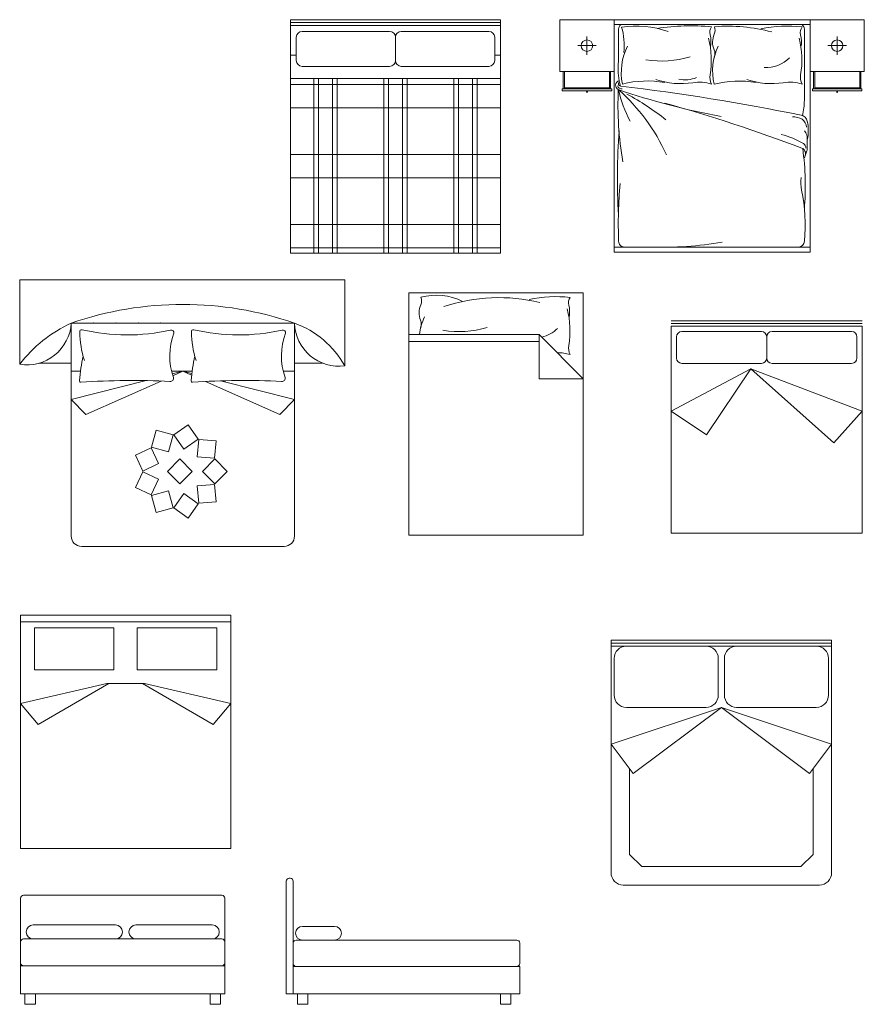
# Model space of a CAD drawing. Units: inches. Extents: x 1994 to 3075, y 3517 to 3950.
# Tile 5 of 58: x 1993.694 to 1993.9789, y 3553.5515 to 3553.8837. Entities that reach past the tile are written whole.
import ezdxf

# ---------------------------------------------------------------- set-up
doc = ezdxf.new("R2010")
doc.units = ezdxf.units.IN
doc.layers.add('A-FURN-REFR', color=8, linetype='Continuous', lineweight=13)

msp = doc.modelspace()

# ---------------------------------------------------------------- linework, layer by layer
at = {"layer": 'A-FURN-REFR'}
for p, q in [((1993.856202557817, 3553.883733619688), (1993.785336416085, 3553.883733619688)), ((1993.785336416085, 3553.804993462208), (1993.785336416085, 3553.883733619688)), ((1993.785336416085, 3553.882749367719), (1993.856202557817, 3553.882749367719)), ((1993.785336416085, 3553.881765115751), (1993.856202557817, 3553.881765115751)), ((1993.856202557817, 3553.883733619688), (1993.856202557817, 3553.804993462208)), ((1993.876219255827, 3553.866219817953), (1993.876219255827, 3553.883730063468)), ((1993.876219255827, 3553.883730063468), (1993.894507734482, 3553.883730063468)), ((1993.894507734482, 3553.883730063474), (1993.960657550884, 3553.883730063461)), ((1993.894507734482, 3553.883730063474), (1993.894507734466, 3553.805323075211)), ((1993.894507734482, 3553.882056862236), (1993.960657550883, 3553.882056862222)), ((1993.960657550884, 3553.883730063461), (1993.960657550867, 3553.805323075197)), ((1993.978946029539, 3553.883730063468), (1993.960657550884, 3553.883730063468)), ((1993.978946029539, 3553.866219817953), (1993.978946029539, 3553.883730063468)), ((1993.787304920022, 3553.869954092129), (1993.787304920022, 3553.877828107877)), ((1993.789273423959, 3553.879796611814), (1993.818800983014, 3553.879796611814)), ((1993.820769486951, 3553.869954092129), (1993.820769486951, 3553.877828107877)), ((1993.822737990888, 3553.879796611814), (1993.852265549944, 3553.879796611814)), ((1993.85423405388, 3553.877828107877), (1993.85423405388, 3553.869954092129)), ((1993.885363495152, 3553.871862008174), (1993.885363495152, 3553.878087873247)), ((1993.958711968042, 3553.85654949402), (1993.958711968047, 3553.880500395955)), ((1993.969801790214, 3553.871862008174), (1993.969801790214, 3553.878087873247)), ((1993.882250562615, 3553.87497494071), (1993.888476427688, 3553.87497494071)), ((1993.97291472275, 3553.87497494071), (1993.966688857678, 3553.87497494071)), ((1993.785336416085, 3553.871779066532), (1993.787304920022, 3553.871779066532)), ((1993.85423405388, 3553.871779066532), (1993.856202557817, 3553.871779066532)), ((1993.789273423959, 3553.867985588192), (1993.818800983014, 3553.867985588192)), ((1993.822737990888, 3553.867985588192), (1993.852265549944, 3553.867985588192)), ((1993.894507734479, 3553.86621981795), (1993.876219255827, 3553.866219817953)), ((1993.877386605528, 3553.866219817953), (1993.877386605527, 3553.860383069447)), ((1993.877775722095, 3553.866219817953), (1993.877775722094, 3553.860383069447)), ((1993.89295126821, 3553.86621981795), (1993.892951268209, 3553.860383069443)), ((1993.893340384778, 3553.86621981795), (1993.893340384776, 3553.860383069443)), ((1993.960657550887, 3553.86621981795), (1993.978946029539, 3553.866219817953)), ((1993.961824900588, 3553.86621981795), (1993.961824900589, 3553.860383069443)), ((1993.962214017155, 3553.86621981795), (1993.962214017156, 3553.860383069443)), ((1993.977389563271, 3553.866219817953), (1993.977389563272, 3553.860383069447)), ((1993.977778679838, 3553.866219817953), (1993.977778679839, 3553.860383069447)), ((1993.785336416085, 3553.863879360431), (1993.856202557817, 3553.863879360431)), ((1993.785336416085, 3553.861910856494), (1993.856202557817, 3553.861910856494)), ((1993.793210431833, 3553.863879360431), (1993.793210431833, 3553.804993462208)), ((1993.794785234983, 3553.863879360431), (1993.794785234983, 3553.804993462208)), ((1993.799509644432, 3553.863879360431), (1993.799509644432, 3553.804993462208)), ((1993.801084447581, 3553.863879360431), (1993.801084447581, 3553.804993462208)), ((1993.816832479078, 3553.863879360431), (1993.816832479078, 3553.804993462208)), ((1993.818407282227, 3553.863879360431), (1993.818407282227, 3553.804993462208)), ((1993.823131691676, 3553.863879360431), (1993.823131691676, 3553.804993462208)), ((1993.824706494825, 3553.863879360431), (1993.824706494825, 3553.804993462208)), ((1993.840454526321, 3553.863879360431), (1993.840454526321, 3553.804993462208)), ((1993.842029329471, 3553.863879360431), (1993.842029329471, 3553.804993462208)), ((1993.84675373892, 3553.863879360431), (1993.84675373892, 3553.804993462208)), ((1993.848328542069, 3553.863879360431), (1993.848328542069, 3553.804993462208)), ((1993.893729501343, 3553.860383069443), (1993.876997488959, 3553.860383069447)), ((1993.876997488959, 3553.860383069447), (1993.876997488959, 3553.859682659626)), ((1993.876997488959, 3553.859682659626), (1993.893729501343, 3553.859682659623)), ((1993.877775722094, 3553.860772186014), (1993.892951268209, 3553.86077218601)), ((1993.893729501343, 3553.859682659623), (1993.893729501343, 3553.860383069443)), ((1993.961435784022, 3553.860383069443), (1993.978167796406, 3553.860383069447)), ((1993.961435784022, 3553.859682659623), (1993.961435784022, 3553.860383069443)), ((1993.978167796406, 3553.859682659626), (1993.961435784022, 3553.859682659623)), ((1993.977389563272, 3553.860772186014), (1993.962214017156, 3553.86077218601)), ((1993.978167796406, 3553.860383069447), (1993.978167796406, 3553.859682659626)), ((1993.785336416085, 3553.854036840746), (1993.856202557817, 3553.854036840746)), ((1993.959684759457, 3553.840101857006), (1993.959684759457, 3553.843919683994)), ((1993.785336416085, 3553.83828880925), (1993.856202557817, 3553.83828880925)), ((1993.959564553778, 3553.83942858826), (1993.958711968038, 3553.83711704396)), ((1993.785336416085, 3553.830414793502), (1993.856202557817, 3553.830414793502)), ((1993.785336416085, 3553.814666762006), (1993.856202557817, 3553.814666762006)), ((1993.785336416085, 3553.806792746258), (1993.856202557817, 3553.806792746258)), ((1993.856202557817, 3553.804993462208), (1993.785336416085, 3553.804993462208)), ((1993.894507734466, 3553.806996276449), (1993.960657550868, 3553.806996276435)), ((1993.894507734466, 3553.805323075211), (1993.960657550867, 3553.805323075197)), ((1993.693977196263, 3553.795927324173), (1993.693977196263, 3553.767437960728)), ((1993.80365945686, 3553.795927324173), (1993.693977196263, 3553.795927324173)), ((1993.80365945686, 3553.795927324173), (1993.80365945686, 3553.76692621804)), ((1993.825218431411, 3553.70978992263), (1993.825218431411, 3553.791608082631)), ((1993.825218431411, 3553.791608082631), (1993.884127555047, 3553.791608082631)), ((1993.884127555047, 3553.791608082631), (1993.884127555047, 3553.70978992263)), ((1993.711353319426, 3553.781334854554), (1993.749029293889, 3553.781334854554)), ((1993.711353319426, 3553.76692621804), (1993.711353319426, 3553.781334854554)), ((1993.786705268352, 3553.781334854554), (1993.749029293889, 3553.781334854554)), ((1993.786705268352, 3553.76692621804), (1993.786705268352, 3553.781334854554)), ((1993.80365945686, 3553.781334854554), (1993.80365945686, 3553.76692621804)), ((1993.978241546912, 3553.782070903671), (1993.913817781701, 3553.782070903671)), ((1993.913817781701, 3553.781176129155), (1993.978241546912, 3553.781176129155)), ((1993.913817781701, 3553.780281354637), (1993.978241546912, 3553.780281354637)), ((1993.913817781701, 3553.710488942325), (1993.913817781701, 3553.780281354637)), ((1993.917396879768, 3553.778491805604), (1993.944240115272, 3553.778491805604)), ((1993.94781921334, 3553.778491805604), (1993.974662448844, 3553.778491805604)), ((1993.978241546912, 3553.780281354637), (1993.978241546912, 3553.710488942325)), ((1993.825218431411, 3553.777469900813), (1993.869203918684, 3553.777469900813)), ((1993.869203918684, 3553.775113537176), (1993.825218431411, 3553.775113537176)), ((1993.884127555047, 3553.762546264449), (1993.869203918684, 3553.777469900813)), ((1993.869203918684, 3553.777469900813), (1993.869203918684, 3553.762546264449)), ((1993.915607330734, 3553.769544060435), (1993.915607330734, 3553.77670225657)), ((1993.946029664306, 3553.769544060435), (1993.946029664306, 3553.77670225657)), ((1993.976451997878, 3553.77670225657), (1993.976451997878, 3553.769544060435)), ((1993.700693126714, 3553.767864459417), (1993.711353319426, 3553.767864459417)), ((1993.711353319426, 3553.709531369957), (1993.711353319426, 3553.76692621804)), ((1993.711353319426, 3553.76507068463), (1993.714474286442, 3553.76507068463)), ((1993.745229054011, 3553.76507068463), (1993.749029293889, 3553.76507068463)), ((1993.749029293889, 3553.76507068463), (1993.74546816915, 3553.764171920895)), ((1993.749029293889, 3553.76507068463), (1993.745653350489, 3553.763563244933)), ((1993.752150260905, 3553.76507068463), (1993.749029293889, 3553.76507068463)), ((1993.749029293889, 3553.76507068463), (1993.752054974805, 3553.764307057271)), ((1993.749029293889, 3553.76507068463), (1993.751991106552, 3553.76374816424)), ((1993.786705268352, 3553.76507068463), (1993.782905028474, 3553.76507068463)), ((1993.786705268352, 3553.767864459417), (1993.796105996925, 3553.767864459417)), ((1993.786705268352, 3553.709531369957), (1993.786705268352, 3553.76692621804)), ((1993.913817781701, 3553.751648570099), (1993.940661017205, 3553.765964962368)), ((1993.917396879768, 3553.767754511401), (1993.944240115272, 3553.767754511401)), ((1993.925706827183, 3553.743673002087), (1993.940661017205, 3553.765964962368)), ((1993.940661017205, 3553.765964962368), (1993.978241546912, 3553.751648570099)), ((1993.940661017205, 3553.765964962368), (1993.968716184927, 3553.740960887158)), ((1993.94781921334, 3553.767754511401), (1993.974662448844, 3553.767754511401)), ((1993.736595982811, 3553.761932740884), (1993.71134319232, 3553.755559391458)), ((1993.741709056693, 3553.761802023153), (1993.716317016293, 3553.750463868108)), ((1993.756653216091, 3553.761666420514), (1993.781741571484, 3553.750463868108)), ((1993.76175885485, 3553.76185797275), (1993.786715395458, 3553.755559391458)), ((1993.869203918684, 3553.762546264449), (1993.884127555047, 3553.762546264449)), ((1993.716317016293, 3553.750463868108), (1993.711353319426, 3553.755561947358)), ((1993.781741571484, 3553.750463868108), (1993.786705268352, 3553.755561947358)), ((1993.913817781701, 3553.751648570099), (1993.925706827183, 3553.743673002087)), ((1993.968716184927, 3553.740960887158), (1993.978241546912, 3553.751648570099)), ((1993.740025946507, 3553.745164882081), (1993.738497487579, 3553.739460595705)), ((1993.745730232882, 3553.743636423153), (1993.740025946507, 3553.745164882081)), ((1993.750795459597, 3553.747063837807), (1993.745957947524, 3553.743676575388)), ((1993.754182722016, 3553.742226325735), (1993.750795459597, 3553.747063837807)), ((1993.744201773955, 3553.737932136777), (1993.745730232882, 3553.743636423153)), ((1993.745957947524, 3553.743676575388), (1993.749345209943, 3553.738839063316)), ((1993.749345209943, 3553.738839063316), (1993.754182722016, 3553.742226325735)), ((1993.754382970911, 3553.742110711981), (1993.753868271643, 3553.736227672426)), ((1993.760266010467, 3553.741596012713), (1993.754382970911, 3553.742110711981)), ((1993.759751311199, 3553.735712973157), (1993.760266010467, 3553.741596012713)), ((1993.738348857402, 3553.739283465158), (1993.732996646062, 3553.736787688022)), ((1993.740844634539, 3553.733931253817), (1993.738348857402, 3553.739283465158)), ((1993.738497487579, 3553.739460595705), (1993.744201773955, 3553.737932136777)), ((1993.732996646062, 3553.736787688022), (1993.735492423198, 3553.731435476681)), ((1993.748019372042, 3553.735495690375), (1993.743843544594, 3553.731319862927)), ((1993.75219519949, 3553.731319862927), (1993.748019372042, 3553.735495690375)), ((1993.753868271643, 3553.736227672426), (1993.759751311199, 3553.735712973157)), ((1993.759830395664, 3553.735495690375), (1993.755654568216, 3553.731319862927)), ((1993.764006223112, 3553.731319862927), (1993.759830395664, 3553.735495690375)), ((1993.735492423198, 3553.731435476681), (1993.740844634539, 3553.733931253817)), ((1993.735492423198, 3553.731204249174), (1993.732996646062, 3553.725852037833)), ((1993.740844634539, 3553.728708472038), (1993.735492423198, 3553.731204249174)), ((1993.738348857402, 3553.723356260697), (1993.740844634539, 3553.728708472038)), ((1993.743843544594, 3553.731319862927), (1993.748019372042, 3553.727144035479)), ((1993.748019372042, 3553.727144035479), (1993.75219519949, 3553.731319862927)), ((1993.755654568216, 3553.731319862927), (1993.759830395664, 3553.727144035479)), ((1993.759830395664, 3553.727144035479), (1993.764006223112, 3553.731319862927)), ((1993.732996646062, 3553.725852037833), (1993.738348857402, 3553.723356260697)), ((1993.759751311199, 3553.726926752697), (1993.753868271643, 3553.72641205343)), ((1993.753868271643, 3553.72641205343), (1993.754382970911, 3553.720529013874)), ((1993.760266010467, 3553.721043713141), (1993.759751311199, 3553.726926752697)), ((1993.744201773955, 3553.724707589078), (1993.738497487579, 3553.72317913015)), ((1993.738497487579, 3553.72317913015), (1993.740025946507, 3553.717474843774)), ((1993.745730232882, 3553.719003302702), (1993.744201773955, 3553.724707589078)), ((1993.749345209943, 3553.72380066254), (1993.745957947524, 3553.718963150467)), ((1993.754182722016, 3553.72041340012), (1993.749345209943, 3553.72380066254)), ((1993.740025946507, 3553.717474843774), (1993.745730232882, 3553.719003302702)), ((1993.745957947524, 3553.718963150467), (1993.750795459597, 3553.715575888047)), ((1993.750795459597, 3553.715575888047), (1993.754182722016, 3553.72041340012)), ((1993.754382970911, 3553.720529013874), (1993.760266010467, 3553.721043713141)), ((1993.884127555047, 3553.70978992263), (1993.825218431411, 3553.70978992263)), ((1993.978241546912, 3553.710488942325), (1993.913817781701, 3553.710488942325)), ((1993.749029293889, 3553.705982905628), (1993.714901783755, 3553.705982905628)), ((1993.749029293889, 3553.705982905628), (1993.783156804023, 3553.705982905628)), ((1993.694294397315, 3553.680492490697), (1993.694294397315, 3553.604071802282)), ((1993.765160539047, 3553.680492490697), (1993.694294397315, 3553.680492490697)), ((1993.765160539047, 3553.604071802282), (1993.765160539047, 3553.680492490697)), ((1993.893506310584, 3553.674395990853), (1993.967915759402, 3553.674395990853)), ((1993.893506310584, 3553.674395990853), (1993.893506310584, 3553.659927486916)), ((1993.893506310584, 3553.67232906172), (1993.893506310584, 3553.674395990853)), ((1993.893506310584, 3553.673362526286), (1993.967915759402, 3553.673362526286)), ((1993.893506310584, 3553.67232906172), (1993.967915759402, 3553.67232906172)), ((1993.893506310584, 3553.67232906172), (1993.893506310584, 3553.651659770381)), ((1993.893506310584, 3553.651659770381), (1993.893506310584, 3553.67232906172)), ((1993.897640168851, 3553.67232906172), (1993.926577176725, 3553.67232906172)), ((1993.963781901135, 3553.67232906172), (1993.934844893261, 3553.67232906172)), ((1993.967915759402, 3553.674395990853), (1993.967915759402, 3553.659927486916)), ((1993.967915759402, 3553.674395990853), (1993.967915759402, 3553.657860557783)), ((1993.967915759402, 3553.674395990853), (1993.967915759402, 3553.67232906172)), ((1993.967915759402, 3553.67232906172), (1993.967915759402, 3553.651659770381)), ((1993.893506310584, 3553.668195203452), (1993.893506310584, 3553.655793628649)), ((1993.89453977515, 3553.668195203452), (1993.89453977515, 3553.655793628649)), ((1993.929677570426, 3553.655793628649), (1993.929677570426, 3553.668195203452)), ((1993.93174449956, 3553.668195203452), (1993.93174449956, 3553.655793628649)), ((1993.966882294835, 3553.668195203452), (1993.966882294835, 3553.655793628649)), ((1993.967915759402, 3553.655793628649), (1993.967915759402, 3553.668195203452)), ((1993.694294397315, 3553.652933435579), (1993.723325541173, 3553.659719936741)), ((1993.724092496647, 3553.659719936741), (1993.700199909126, 3553.645846821406)), ((1993.723325541173, 3553.659719936741), (1993.736129395189, 3553.659719936741)), ((1993.735362439715, 3553.659719936741), (1993.759255027236, 3553.645846821406)), ((1993.765160539047, 3553.652933435579), (1993.736129395189, 3553.659719936741)), ((1993.700199909126, 3553.645846821406), (1993.694294397315, 3553.652933435579)), ((1993.759255027236, 3553.645846821406), (1993.765160539047, 3553.652933435579)), ((1993.893506310584, 3553.639258195577), (1993.930711034993, 3553.651659770381)), ((1993.893506310584, 3553.639258195577), (1993.930711034993, 3553.651659770381)), ((1993.893506310584, 3553.651659770381), (1993.893506310584, 3553.639258195577)), ((1993.893506310584, 3553.639258195577), (1993.893506310584, 3553.651659770381)), ((1993.898673633418, 3553.651659770381), (1993.925543712158, 3553.651659770381)), ((1993.900947255465, 3553.629336935735), (1993.930711034993, 3553.651659770381)), ((1993.960474814521, 3553.629336935735), (1993.930711034993, 3553.651659770381)), ((1993.967915759402, 3553.639258195577), (1993.930711034993, 3553.651659770381)), ((1993.967915759402, 3553.639258195577), (1993.930711034993, 3553.651659770381)), ((1993.935878357827, 3553.651659770381), (1993.962748436568, 3553.651659770381)), ((1993.967915759402, 3553.653726699515), (1993.967915759402, 3553.595852683767)), ((1993.893506310584, 3553.641325124711), (1993.893506310584, 3553.595852683767)), ((1993.900947255465, 3553.629336935735), (1993.893506310584, 3553.639258195577)), ((1993.893506310584, 3553.639258195577), (1993.900947255465, 3553.629336935735)), ((1993.967915759402, 3553.639258195577), (1993.960474814521, 3553.629336935735)), ((1993.960474814521, 3553.629336935735), (1993.967915759402, 3553.639258195577)), ((1993.899707097985, 3553.630990479042), (1993.899707097985, 3553.602053471168)), ((1993.961714972001, 3553.630990479042), (1993.961714972001, 3553.602053471168)), ((1993.694294397315, 3553.604071802282), (1993.765160539047, 3553.604071802282)), ((1993.903840956253, 3553.597919612901), (1993.899707097985, 3553.602053471168)), ((1993.957581113733, 3553.597919612901), (1993.961714972001, 3553.602053471168)), ((1993.903840956253, 3553.597919612901), (1993.957581113733, 3553.597919612901)), ((1993.783929377259, 3553.593027229099), (1993.783929377259, 3553.554949278618)), ((1993.784895822703, 3553.593993674543), (1993.78528240088, 3553.593993674543)), ((1993.786248846324, 3553.593027229099), (1993.786248846324, 3553.554949278618)), ((1993.897640168851, 3553.591718825499), (1993.963781901135, 3553.591718825499)), ((1993.694294397315, 3553.555013382106), (1993.694294397315, 3553.587263222953)), ((1993.762207783142, 3553.588247474922), (1993.695278649283, 3553.588247474922)), ((1993.76319203511, 3553.555013382106), (1993.76319203511, 3553.587263222953)), ((1993.698521984855, 3553.578241728563), (1993.726310788034, 3553.578241728563)), ((1993.75896444757, 3553.578241728563), (1993.733209943662, 3553.578241728563)), ((1993.789370152606, 3553.577757391089), (1993.800194341576, 3553.577757391089)), ((1993.762207783142, 3553.573517319114), (1993.695278649283, 3553.573517319114)), ((1993.733211644699, 3553.573517363929), (1993.733211644699, 3553.573517352119)), ((1993.733211644699, 3553.573517167079), (1993.733211644699, 3553.573517155268)), ((1993.733211648636, 3553.573517367867), (1993.733211711628, 3553.573517367867)), ((1993.733211648636, 3553.573517348181), (1993.733211660447, 3553.573517348181)), ((1993.733211648636, 3553.573517171016), (1993.733211660447, 3553.573517171016)), ((1993.733211648636, 3553.573517151331), (1993.733211711628, 3553.573517151331)), ((1993.733211660447, 3553.573517348181), (1993.733211660447, 3553.573517171016)), ((1993.73321177455, 3553.573517365745), (1993.733211699817, 3553.573517221975)), ((1993.733211699817, 3553.573517348181), (1993.733211699817, 3553.573517221975)), ((1993.733211699817, 3553.573517348181), (1993.733211711628, 3553.573517348181)), ((1993.733211790807, 3553.57351734606), (1993.733211699817, 3553.573517171016)), ((1993.733211699817, 3553.573517171016), (1993.733211711628, 3553.573517171016)), ((1993.733211715565, 3553.573517363929), (1993.733211715565, 3553.573517352119)), ((1993.733211715565, 3553.573517167079), (1993.733211715565, 3553.573517155268)), ((1993.733211757761, 3553.573517167079), (1993.733211757761, 3553.573517155268)), ((1993.733211761698, 3553.573517171016), (1993.733211777446, 3553.573517171016)), ((1993.733211761698, 3553.573517151331), (1993.733211842197, 3553.573517151331)), ((1993.733211828967, 3553.573517270133), (1993.733211777446, 3553.573517171016)), ((1993.733211778043, 3553.573517367867), (1993.73321211117, 3553.573517367867)), ((1993.7332117943, 3553.573517348181), (1993.7332119795, 3553.573517348181)), ((1993.733211809282, 3553.57351728588), (1993.733211809282, 3553.573517274069)), ((1993.733211813219, 3553.573517289817), (1993.733211893718, 3553.573517289817)), ((1993.733211813219, 3553.573517270133), (1993.733211828967, 3553.573517270133)), ((1993.73321187797, 3553.573517270133), (1993.733211826448, 3553.573517171016)), ((1993.733211826448, 3553.573517171016), (1993.733211842197, 3553.573517171016)), ((1993.733211846134, 3553.573517167079), (1993.733211846134, 3553.573517155268)), ((1993.733211867723, 3553.573517167079), (1993.733211867723, 3553.573517155268)), ((1993.73321187166, 3553.573517171016), (1993.733211887407, 3553.573517171016)), ((1993.73321187166, 3553.573517151331), (1993.733212018064, 3553.573517151331)), ((1993.73321187797, 3553.573517270133), (1993.733211893718, 3553.573517270133)), ((1993.7332119795, 3553.573517348181), (1993.733211887407, 3553.573517171016)), ((1993.733211897655, 3553.57351728588), (1993.733211897655, 3553.573517274069)), ((1993.733211986829, 3553.573517268012), (1993.733211939401, 3553.573517176769)), ((1993.733211942894, 3553.573517171016), (1993.733211979294, 3553.573517171016)), ((1993.733212027825, 3553.57351726438), (1993.733211979294, 3553.573517171016)), ((1993.733211990322, 3553.573517270133), (1993.733212024332, 3553.573517270133)), ((1993.7332120274, 3553.57351734606), (1993.733212001155, 3553.57351729557)), ((1993.733212004648, 3553.573517289817), (1993.733212038657, 3553.573517289817)), ((1993.733212081944, 3553.573517274222), (1993.733212018064, 3553.573517151331)), ((1993.733212030893, 3553.573517348181), (1993.733212064902, 3553.573517348181)), ((1993.733212068396, 3553.573517342428), (1993.73321204215, 3553.573517291939)), ((1993.733212135012, 3553.573517283453), (1993.733212075305, 3553.573517168589)), ((1993.733212078451, 3553.573517279975), (1993.733212082544, 3553.573517279975)), ((1993.73321212165, 3553.573517350608), (1993.733212086037, 3553.573517282096)), ((1993.733212085784, 3553.573517151331), (1993.733212163665, 3553.573517151331)), ((1993.733212175987, 3553.573517268012), (1993.733212128559, 3553.573517176769)), ((1993.733212132052, 3553.573517171016), (1993.73321215219, 3553.573517171016)), ((1993.733212145492, 3553.573517289817), (1993.733212223373, 3553.573517289817)), ((1993.733212203112, 3553.57351726438), (1993.733212155684, 3553.573517173138)), ((1993.733212233852, 3553.573517272559), (1993.733212174145, 3553.573517157694)), ((1993.733212179481, 3553.573517270133), (1993.733212199619, 3553.573517270133)), ((1993.787215291767, 3553.573118452959), (1993.861703089296, 3553.573118452959)), ((1993.800196011838, 3553.573118496963), (1993.800196011838, 3553.573118485366)), ((1993.800196011838, 3553.573118303674), (1993.800196011838, 3553.573118292077)), ((1993.800196015704, 3553.573118500829), (1993.800196077557, 3553.573118500829)), ((1993.800196015704, 3553.5731184815), (1993.800196027302, 3553.5731184815)), ((1993.800196015704, 3553.57311830754), (1993.800196027302, 3553.57311830754)), ((1993.800196015704, 3553.57311828821), (1993.800196077557, 3553.57311828821)), ((1993.800196027302, 3553.5731184815), (1993.800196027302, 3553.57311830754)), ((1993.800196139341, 3553.573118498746), (1993.800196065959, 3553.573118357576)), ((1993.800196065959, 3553.5731184815), (1993.800196065959, 3553.573118357576)), ((1993.800196065959, 3553.5731184815), (1993.800196077557, 3553.5731184815)), ((1993.800196155303, 3553.573118479417), (1993.800196065959, 3553.57311830754)), ((1993.800196065959, 3553.57311830754), (1993.800196077557, 3553.57311830754)), ((1993.800196081422, 3553.573118496963), (1993.800196081422, 3553.573118485366)), ((1993.800196081422, 3553.573118303674), (1993.800196081422, 3553.573118292077)), ((1993.800196122855, 3553.573118303674), (1993.800196122855, 3553.573118292077)), ((1993.800196126721, 3553.57311830754), (1993.800196142184, 3553.57311830754)), ((1993.800196126721, 3553.57311828821), (1993.800196205763, 3553.57311828821)), ((1993.800196192773, 3553.573118404863), (1993.800196142184, 3553.57311830754)), ((1993.800196142771, 3553.573118500829), (1993.800196469871, 3553.573118500829)), ((1993.800196158733, 3553.5731184815), (1993.800196340582, 3553.5731184815)), ((1993.800196173444, 3553.573118420326), (1993.800196173444, 3553.573118408729)), ((1993.80019617731, 3553.573118424192), (1993.800196256352, 3553.573118424192)), ((1993.80019617731, 3553.573118404863), (1993.800196192773, 3553.573118404863)), ((1993.80019624089, 3553.573118404863), (1993.8001961903, 3553.57311830754)), ((1993.8001961903, 3553.57311830754), (1993.800196205763, 3553.57311830754)), ((1993.800196209629, 3553.573118303674), (1993.800196209629, 3553.573118292077)), ((1993.800196230827, 3553.573118303674), (1993.800196230827, 3553.573118292077)), ((1993.800196234693, 3553.57311830754), (1993.800196250156, 3553.57311830754)), ((1993.800196234693, 3553.57311828821), (1993.800196378449, 3553.57311828821)), ((1993.80019624089, 3553.573118404863), (1993.800196256352, 3553.573118404863)), ((1993.800196340582, 3553.5731184815), (1993.800196250156, 3553.57311830754)), ((1993.800196260218, 3553.573118420326), (1993.800196260218, 3553.573118408729)), ((1993.800196347779, 3553.573118402781), (1993.800196301209, 3553.573118313189)), ((1993.800196304639, 3553.57311830754), (1993.80019634038, 3553.57311830754)), ((1993.800196388033, 3553.573118399214), (1993.80019634038, 3553.57311830754)), ((1993.800196351209, 3553.573118404863), (1993.800196384603, 3553.573118404863)), ((1993.800196387615, 3553.573118479417), (1993.800196361845, 3553.573118429841)), ((1993.800196365275, 3553.573118424192), (1993.80019639867, 3553.573118424192)), ((1993.800196441173, 3553.573118408878), (1993.800196378449, 3553.57311828821)), ((1993.800196391046, 3553.5731184815), (1993.80019642444, 3553.5731184815)), ((1993.80019642787, 3553.573118475851), (1993.8001964021, 3553.573118426275)), ((1993.800196493281, 3553.573118417943), (1993.800196434654, 3553.573118305158)), ((1993.800196437743, 3553.573118414527), (1993.800196441762, 3553.573118414527)), ((1993.800196480161, 3553.573118483882), (1993.800196445192, 3553.57311841661)), ((1993.800196444944, 3553.57311828821), (1993.800196521416, 3553.57311828821)), ((1993.800196533515, 3553.573118402781), (1993.800196486944, 3553.573118313189)), ((1993.800196490375, 3553.57311830754), (1993.800196510149, 3553.57311830754)), ((1993.800196503571, 3553.573118424192), (1993.800196580043, 3553.573118424192)), ((1993.800196560149, 3553.573118399214), (1993.800196513579, 3553.573118309623)), ((1993.800196590333, 3553.573118407245), (1993.800196531706, 3553.57311829446)), ((1993.800196536945, 3553.573118404863), (1993.800196556719, 3553.573118404863)), ((1993.862669534739, 3553.572152007515), (1993.862669534739, 3553.56519360032)), ((1993.76319203511, 3553.564462201004), (1993.694294397315, 3553.564462201004)), ((1993.786248846324, 3553.564227154877), (1993.861703089296, 3553.564227154877)), ((1993.861703089296, 3553.564227154877), (1993.862669534739, 3553.564227154877)), ((1993.862669534739, 3553.564227154877), (1993.862669534739, 3553.554949278618)), ((1993.76319203511, 3553.555013382106), (1993.694294397315, 3553.555013382106)), ((1993.695746159387, 3553.555013382106), (1993.695746159387, 3553.55147007502)), ((1993.699289466474, 3553.555013382106), (1993.699289466474, 3553.55147007502)), ((1993.758196965951, 3553.555013382106), (1993.758196965951, 3553.55147007502)), ((1993.761740273038, 3553.555013382106), (1993.761740273038, 3553.55147007502)), ((1993.783929377259, 3553.554949278618), (1993.862669534739, 3553.554949278618)), ((1993.787670212685, 3553.554949278618), (1993.787670212685, 3553.55147007502)), ((1993.791149416282, 3553.554949278618), (1993.791149416282, 3553.55147007502)), ((1993.856210386026, 3553.554949278618), (1993.856210386026, 3553.55147007502)), ((1993.859689589623, 3553.554949278618), (1993.859689589623, 3553.55147007502)), ((1993.699289466474, 3553.55147007502), (1993.695746159387, 3553.55147007502)), ((1993.761740273038, 3553.55147007502), (1993.758196965951, 3553.55147007502)), ((1993.791149416282, 3553.55147007502), (1993.787670212685, 3553.55147007502)), ((1993.859689589623, 3553.55147007502), (1993.856210386026, 3553.55147007502))]:
    msp.add_line(p, q, dxfattribs=at)
for points in [[(1993.694294397315, 3553.682811959762), (1993.765160539047, 3553.682811959762), (1993.765160539047, 3553.680492490697), (1993.694294397315, 3553.680492490697)], [(1993.725790460307, 3553.67852398676), (1993.725790460307, 3553.664350758414), (1993.699018806764, 3553.664350758414), (1993.699018806764, 3553.67852398676)], [(1993.760436129598, 3553.67852398676), (1993.760436129598, 3553.664350758414), (1993.733664476055, 3553.664350758414), (1993.733664476055, 3553.67852398676)]]:
    msp.add_lwpolyline(points, close=True, dxfattribs=at)
for centre in [(1993.885363495152, 3553.87497494071), (1993.969801790214, 3553.87497494071)]:
    msp.add_circle(centre, 0.0019455828353276, dxfattribs=at)
for centre, radius, start, end in [((1993.898009783585, 3553.880500395968), 0.0019455828353276, 126.8698976337993, 179.9999999880876), ((1993.901750451541, 3553.847780504995), 0.0338061826761343, 71.0292396466785, 98.01463022582239), ((1993.877854489022, 3553.875318848574), 0.0200804373013914, 352.4610811587552, 17.19907473199907), ((1993.92025362591, 3553.809706760066), 0.071952262989263, 84.30946080187233, 98.94135126792816), ((1993.92991413471, 3553.879494548308), 0.0031075126812102, 144.3787648229011, 195.1987658355305), ((1993.925413987735, 3553.880175337851), 0.0032028341489732, 335.7877323280015, 21.71237864400314), ((1993.933001918543, 3553.82504237093), 0.0565064023996118, 74.89247536308716, 94.681970907379), ((1993.952981615313, 3553.840133134688), 0.0414680575843914, 83.14136388124066, 102.4247502365447), ((1993.960459785224, 3553.879494548301), 0.0031075126812102, 144.3787648229011, 195.1987658355305), ((1993.956766385212, 3553.880500395955), 0.0019455828353276, 359.9999999880876, 53.13010234330246), ((1993.789273423959, 3553.877828107877), 0.0019685039370079, 90, 180), ((1993.818800983014, 3553.877828107877), 0.0019685039370079, 0, 90), ((1993.822737990888, 3553.877828107877), 0.0019685039370079, 90, 180), ((1993.852265549944, 3553.877828107877), 0.0019685039370079, 0, 90), ((1993.358445808769, 3553.879659393653), 0.5376190497749752, 358.8114973710085, 0.0896283401223897), ((1993.918619716838, 3553.87642618413), 0.0085962787467616, 347.311957921453, 15.19876583553051), ((1993.934333027161, 3553.876164667004), 0.0065764677133891, 155.7877323280015, 202.8808293159797), ((1993.949165367353, 3553.876426184124), 0.0085962787467616, 347.311957921453, 15.19876583553051), ((1993.916703077656, 3553.865885545193), 0.0197598411462801, 153.3318705081994, 191.2891230798232), ((1993.897480114389, 3553.870112338171), 0.0298558147000044, 350.3711224665587, 14.25995084780135), ((1993.947600168964, 3553.866401437366), 0.0198519972069101, 155.1179531461462, 192.9861889591517), ((1993.928025764904, 3553.870112338164), 0.0298558147000044, 350.3711224665587, 14.25995084780135), ((1993.910625880842, 3553.902002055843), 0.0322267158934928, 260.4320326468418, 287.2701993260345), ((1993.925196658872, 3553.872308915851), 0.0033401870886801, 339.0160855821216, 22.88082931597971), ((1993.789273423959, 3553.869954092129), 0.0019685039370079, 180, 270), ((1993.818800983014, 3553.869954092129), 0.0019685039370079, 270, 0), ((1993.822737990888, 3553.869954092129), 0.0019685039370079, 180, 270), ((1993.852265549944, 3553.869954092129), 0.0019685039370079, 270, 0), ((1993.915922083087, 3553.866780256404), 0.0200474922626186, 175.0553728283678, 195.8557099358243), ((1993.945594092227, 3553.878993118354), 0.0114567055564695, 267.8294752673963, 315.0098308273483), ((1993.93184101892, 3553.864282811066), 0.004996088352876, 170.3711224665586, 206.9649370961853), ((1993.962386669434, 3553.86428281106), 0.004996088352876, 170.3711224665586, 206.9649370961853), ((1993.89665736009, 3553.861608001213), 0.0016105685091622, 106.3004786234319, 243.938180591863), ((1993.89712536313, 3553.861994480702), 0.0016095821071006, 202.6051908922757, 274.4988817166678), ((1993.896804607686, 3553.862098460906), 0.0008128892221172, 129.3957755051945, 258.1255955891823), ((1993.81019279453, 3553.128525293408), 0.737858914858732, 78.47703152821846, 83.27200853442297), ((1993.905750797334, 3553.828477165661), 0.034582210914614, 80.14382640862489, 104.1008515969175), ((1993.916980157655, 3553.887548683202), 0.0254057342932298, 250.6572032486362, 279.2500666033769), ((1993.918565466571, 3553.873432520417), 0.009989213432703, 257.148031947205, 292.3825063085086), ((1993.923277616005, 3553.849091026485), 0.0135641447689492, 72.35976010254194, 99.39258996595309), ((1993.936748413801, 3553.829330842628), 0.0336972432594088, 80.32657587842615, 104.5973118255227), ((1993.947588563615, 3553.886782064937), 0.0246390736856652, 250.3559327023518, 279.3925899659531), ((1993.953823266519, 3553.849091026479), 0.0135641447689492, 72.35976010254194, 99.39258996595309), ((1993.885363495151, 3553.859365161903), 0.00014591871265, 359.9999999880876, 179.9999999880876), ((1993.885363495151, 3553.859365161903), 0.00014591871265, 179.9999999880876, 359.9999999880876), ((1994.01246655477, 3553.855061882958), 0.1166283141987217, 177.4940716817132, 189.5094068679036), ((1993.852479390668, 3553.81110757628), 0.065543355857517, 24.38326925012849, 48.45324971012612), ((1993.97268618661, 3554.08298035195), 0.2356625857026807, 250.9968676421653, 259.7279623061984), ((1993.948388902922, 3553.873419997887), 0.0540893550839264, 194.1893851607317, 206.3095844034524), ((1993.860498342266, 3553.786181436841), 0.0819509525067612, 51.03759283326017, 62.08562985249065), ((1993.969801790214, 3553.859365161903), 0.00014591871265, 1.19123935e-08, 180.0000000119124), ((1993.969801790214, 3553.859365161903), 0.00014591871265, 180.0000000119124, 1.19123935e-08), ((1993.768392853046, 3553.342085543028), 0.5331120127502642, 69.18683318772709, 74.4079909335134), ((1993.933994671555, 3553.856881132545), 0.0247195212287987, 347.0890423172248, 359.2312934508153), ((1993.957039730783, 3553.848844386526), 0.0027238159694586, 12.88269036848606, 78.38686031445394), ((1993.954149482791, 3553.841873463306), 0.0091331594194461, 65.03385580996276, 86.4640048798947), ((1993.955502491585, 3553.847107458108), 0.0039416012902181, 4.684898432501862, 50.59840531545589), ((1993.946214875293, 3553.846368605261), 0.013828183994568, 346.9286456497866, 12.88269036848606), ((1994.112435388242, 3553.829987895742), 0.2168115609509192, 175.697202442643, 183.2229785434103), ((1993.945364263942, 3553.821064079928), 0.0245737753138132, 58.01122975656369, 76.86512646864662), ((1993.955497571437, 3553.843671043124), 0.0041945638393764, 356.601689895136, 37.73019638534235), ((1993.957499790994, 3553.840420208836), 0.001728440251783, 359.0101027185217, 59.29760239232226), ((1993.957175235246, 3553.838572889993), 0.0019455828353276, 339.7541012352643, 70.67241641354788), ((1993.8658633368, 3553.827480032637), 0.0931787946855045, 355.1752823324409, 7.876466900264919), ((1993.957739176622, 3553.840101857006), 0.0019455828353276, 339.7541012352643, 359.9999999880876), ((1993.957739176622, 3553.840101857006), 0.0019455828353276, 339.7541012352643, 359.9999999880876), ((1994.037227235995, 3553.81492375444), 0.1412897221787423, 174.5126540947314, 182.4265021931356), ((1993.970531111008, 3553.828766420453), 0.0129749866847535, 172.4746658505032, 191.3425348756069), ((1993.89943294368, 3553.814504707719), 0.0595394659951302, 354.6389628949611, 11.34253487560691), ((1993.898009783571, 3553.808941859284), 0.0019455828353276, 179.9999999880876, 269.9999999880876), ((1993.910552260072, 3553.931082183793), 0.1241401229318277, 268.3066004926072, 279.4831521227457), ((1993.956766385197, 3553.808941859271), 0.0019455828353276, 269.9999999880876, 359.9999999880876), ((1993.826365191638, 3553.788859136397), 0.0032028341489732, 335.7877323280015, 21.71237864400314), ((1993.834571482331, 3553.771000619215), 0.0197486987265365, 63.38196750841395, 105.3587807882128), ((1993.855629813965, 3553.731269192068), 0.0586716085832465, 76.33335198625635, 108.4694926903225), ((1993.874744665, 3553.748816933235), 0.0414680575843914, 83.14136388124066, 102.4247502365447), ((1993.882222834911, 3553.788178346849), 0.0031075126812102, 144.3787648229011, 195.1987658355305), ((1993.749029293889, 3553.672242630522), 0.1154148707744014, 70.94718958950003, 109.0528104105), ((1993.835284231064, 3553.78484846555), 0.0065764677133891, 155.7877323280015, 202.8808293159797), ((1993.849788814591, 3553.778796136711), 0.0298558147000044, 350.3711224665587, 14.25995084780135), ((1993.87092841704, 3553.785109982671), 0.0085962787467616, 347.311957921453, 15.19876583553051), ((1993.696410805833, 3553.782206725607), 0.0149679280998906, 260.6428391444751, 356.6606718254233), ((1993.73105315447, 3553.73889131109), 0.0467924981438534, 114.8979987522044, 142.4055122176543), ((1993.80166713012, 3553.781760957868), 0.0149679280998906, 181.6313026200066, 277.6491353005932), ((1993.77594799475, 3553.751498061797), 0.031716764294517, 29.10655736921449, 70.17388055115411), ((1993.848551372867, 3553.775085235913), 0.0198519972069101, 155.1179531461462, 173.1008468379609), ((1993.826147862774, 3553.780992714397), 0.0033401870886801, 339.0160855821216, 22.88082931597971), ((1993.714870183368, 3553.778487848543), 0.0006418505258738, 76.75528123471223, 195.8617738841529), ((1993.747129956518, 3553.778699553211), 0.0328794636929712, 180.6746350066927, 197.6150049639686), ((1993.730229777517, 3553.84374467344), 0.06639821457078, 256.7552812347122, 282.7325392847955), ((1993.766776185203, 3553.770322086022), 0.0221778285498265, 159.8977315978536, 199.2109654929595), ((1993.745129520674, 3553.778171112833), 0.0008506260458002, 344.5519607965242, 108.1917532780373), ((1993.752546157831, 3553.778487848543), 0.0006418505258738, 76.75528123471223, 195.8617738841529), ((1993.784805930981, 3553.778699553211), 0.0328794636929712, 180.6746350066927, 197.6150049639686), ((1993.76790575198, 3553.84374467344), 0.06639821457078, 256.7552812347122, 282.7325392847955), ((1993.804452159666, 3553.770322086022), 0.0221778285498265, 159.8977315978536, 199.2109654929595), ((1993.782805495137, 3553.778171112833), 0.0008506260458002, 344.5519607965242, 108.1917532780373), ((1993.84212273526, 3553.810685854384), 0.0322267158934928, 260.4320326468418, 287.2701993260345), ((1993.867357141914, 3553.787676916901), 0.0114567055564695, 283.9361364524131, 315.0098308273483), ((1993.917396879768, 3553.77670225657), 0.0017895490336435, 90, 180), ((1993.944240115272, 3553.77670225657), 0.0017895490336435, 0, 90), ((1993.94781921334, 3553.77670225657), 0.0017895490336435, 90, 180), ((1993.974662448844, 3553.77670225657), 0.0017895490336435, 0, 90), ((1993.875586316206, 3553.757774825026), 0.0135641447689492, 72.35976010254194, 91.05260058094025), ((1993.884149719121, 3553.772966609607), 0.004996088352876, 170.3711224665586, 206.9649370961853), ((1993.778242281199, 3553.756725899004), 0.0643116832495532, 167.8842515247495, 175.3339342363999), ((1993.815918255662, 3553.756725899004), 0.0643116832495532, 167.8842515247495, 175.3339342363999), ((1993.917396879768, 3553.769544060435), 0.0017895490336435, 180, 270), ((1993.944240115272, 3553.769544060435), 0.0017895490336435, 270, 0), ((1993.94781921334, 3553.769544060435), 0.0017895490336435, 180, 270), ((1993.974662448844, 3553.769544060435), 0.0017895490336435, 270, 0), ((1993.714544479838, 3553.761837879797), 0.0004182202622219, 163.3743218240804, 282.7732015833482), ((1993.732009157747, 3553.482452053103), 0.2795183246341876, 87.4067690575203, 93.56325965747406), ((1993.744865587792, 3553.762687306557), 0.0010248466488433, 258.1968271318752, 19.21096549295958), ((1993.752220454301, 3553.761837879797), 0.0004182202622219, 163.3743218240804, 282.7732015833482), ((1993.76968513221, 3553.482452053103), 0.2795183246341876, 87.4067690575203, 93.56325965747406), ((1993.782541562255, 3553.762687306557), 0.0010248466488433, 258.1968271318752, 19.21096549295958), ((1993.714901783755, 3553.709531369957), 0.0035484643286817, 180, 270), ((1993.783156804023, 3553.709531369957), 0.0035484643286817, 270, 0), ((1993.898673633418, 3553.668195203452), 0.0041338582677166, 90, 180), ((1993.925543712158, 3553.668195203452), 0.0041338582677166, 0, 90), ((1993.935878357827, 3553.668195203452), 0.0041338582677166, 90, 180), ((1993.962748436568, 3553.668195203452), 0.0041338582677166, 0, 90), ((1993.898673633418, 3553.655793628649), 0.0041338582677166, 180, 270), ((1993.925543712158, 3553.655793628649), 0.0041338582677166, 270, 0), ((1993.935878357827, 3553.655793628649), 0.0041338582677166, 180, 270), ((1993.962748436568, 3553.655793628649), 0.0041338582677166, 270, 0), ((1993.897640168851, 3553.595852683767), 0.0041338582677166, 180, 270), ((1993.963781901135, 3553.595852683767), 0.0041338582677166, 270, 0), ((1993.784895822703, 3553.593027229099), 0.0009664454437014, 90, 180), ((1993.78528240088, 3553.593027229099), 0.0009664454437014, 0, 90), ((1993.695278649283, 3553.587263222953), 0.0009842519685039, 90, 180), ((1993.762207783142, 3553.587263222953), 0.0009842519685039, 0, 90), ((1993.698521984855, 3553.575879523839), 0.0023622047244095, 90, 270), ((1993.726310788034, 3553.575879523839), 0.0023622047244095, 270, 90), ((1993.733209943662, 3553.575879523839), 0.0023622047244095, 90, 270), ((1993.75896444757, 3553.575879523839), 0.0023622047244095, 270, 90), ((1993.789370152606, 3553.575437922024), 0.0023194690648836, 90, 270), ((1993.800194341576, 3553.575437922024), 0.0023194690648836, 270, 90), ((1993.695278649283, 3553.572533067146), 0.0009842519685039, 90, 180), ((1993.733211648636, 3553.573517363929), 3.9370079e-09, 90, 180), ((1993.733211648636, 3553.573517352119), 3.9370079e-09, 180, 270), ((1993.733211648636, 3553.573517167079), 3.9370079e-09, 90, 180), ((1993.733211648636, 3553.573517155268), 3.9370079e-09, 180, 270), ((1993.733211711628, 3553.573517363929), 3.9370079e-09, 0, 90), ((1993.733211711628, 3553.573517352119), 3.9370079e-09, 270, 0), ((1993.733211711628, 3553.573517167079), 3.9370079e-09, 0, 90), ((1993.733211711628, 3553.573517155268), 3.9370079e-09, 270, 0), ((1993.733211761698, 3553.573517167079), 3.9370079e-09, 90, 180), ((1993.733211761698, 3553.573517155268), 3.9370079e-09, 180, 270), ((1993.733211778043, 3553.573517363929), 3.9370079e-09, 90, 152.534173107642), ((1993.7332117943, 3553.573517344244), 3.9370079e-09, 90, 152.534173107642), ((1993.733211813219, 3553.57351728588), 3.9370079e-09, 90, 180), ((1993.733211813219, 3553.573517274069), 3.9370079e-09, 180, 270), ((1993.733211842197, 3553.573517167079), 3.9370079e-09, 0, 90), ((1993.733211842197, 3553.573517155268), 3.9370079e-09, 270, 0), ((1993.73321187166, 3553.573517167079), 3.9370079e-09, 90, 180), ((1993.73321187166, 3553.573517155268), 3.9370079e-09, 180, 270), ((1993.733211893718, 3553.57351728588), 3.9370079e-09, 0, 90), ((1993.733211893718, 3553.573517274069), 3.9370079e-09, 270, 0), ((1993.733211942894, 3553.573517174953), 3.9370079e-09, 152.534173107642, 270), ((1993.733211990322, 3553.573517266195), 3.9370079e-09, 90, 152.534173107642), ((1993.733212004648, 3553.573517293755), 3.9370079e-09, 152.534173107642, 270), ((1993.733212024332, 3553.573517266195), 3.9370079e-09, 332.5341731076421, 90), ((1993.733212030893, 3553.573517344244), 3.9370079e-09, 90, 152.534173107642), ((1993.733212038657, 3553.573517293755), 3.9370079e-09, 270, 332.5341731076421), ((1993.733212064902, 3553.573517344244), 3.9370079e-09, 332.5341731076421, 90), ((1993.733212085784, 3553.573517163142), 1.18110236e-08, 152.534173107642, 270), ((1993.733212078451, 3553.573517276038), 3.9370079e-09, 332.5341731076421, 90), ((1993.733212082544, 3553.573517283912), 3.9370079e-09, 270, 332.5341731076421), ((1993.73321211117, 3553.573517356055), 1.18110236e-08, 332.5341731076421, 90), ((1993.733212132052, 3553.573517174953), 3.9370079e-09, 152.534173107642, 270), ((1993.733212145492, 3553.573517278006), 1.18110236e-08, 90, 152.534173107642), ((1993.73321215219, 3553.573517174953), 3.9370079e-09, 270, 332.5341731076421), ((1993.733212163665, 3553.573517163142), 1.18110236e-08, 270, 332.5341731076421), ((1993.733212179481, 3553.573517266195), 3.9370079e-09, 90, 152.534173107642), ((1993.733212199619, 3553.573517266195), 3.9370079e-09, 332.5341731076421, 90), ((1993.733212223373, 3553.573517278006), 1.18110236e-08, 332.5341731076421, 90), ((1993.762207783142, 3553.572533067146), 0.0009842519685039, 0, 90), ((1993.787215291767, 3553.572152007515), 0.0009664454437014, 90, 180), ((1993.800196015704, 3553.573118496963), 3.8657818e-09, 90, 180), ((1993.800196015704, 3553.573118485366), 3.8657818e-09, 180, 270), ((1993.800196015704, 3553.573118303674), 3.8657818e-09, 90, 180), ((1993.800196015704, 3553.573118292077), 3.8657818e-09, 180, 270), ((1993.800196077557, 3553.573118496963), 3.8657818e-09, 0, 90), ((1993.800196077557, 3553.573118485366), 3.8657818e-09, 270, 0), ((1993.800196077557, 3553.573118303674), 3.8657818e-09, 0, 90), ((1993.800196077557, 3553.573118292077), 3.8657818e-09, 270, 0), ((1993.800196126721, 3553.573118303674), 3.8657818e-09, 90, 180), ((1993.800196126721, 3553.573118292077), 3.8657818e-09, 180, 270), ((1993.800196142771, 3553.573118496963), 3.8657818e-09, 90, 152.534173107642), ((1993.800196158733, 3553.573118477635), 3.8657818e-09, 90, 152.534173107642), ((1993.80019617731, 3553.573118420326), 3.8657818e-09, 90, 180), ((1993.80019617731, 3553.573118408729), 3.8657818e-09, 180, 270), ((1993.800196205763, 3553.573118303674), 3.8657818e-09, 0, 90), ((1993.800196205763, 3553.573118292077), 3.8657818e-09, 270, 0), ((1993.800196234693, 3553.573118303674), 3.8657818e-09, 90, 180), ((1993.800196234693, 3553.573118292077), 3.8657818e-09, 180, 270), ((1993.800196256352, 3553.573118420326), 3.8657818e-09, 0, 90), ((1993.800196256352, 3553.573118408729), 3.8657818e-09, 270, 0), ((1993.800196304639, 3553.573118311405), 3.8657818e-09, 152.534173107642, 270), ((1993.800196351209, 3553.573118400997), 3.8657818e-09, 90, 152.534173107642), ((1993.800196365275, 3553.573118428058), 3.8657818e-09, 152.534173107642, 270), ((1993.800196384603, 3553.573118400997), 3.8657818e-09, 332.5341731076421, 90), ((1993.800196391046, 3553.573118477635), 3.8657818e-09, 90, 152.534173107642), ((1993.80019639867, 3553.573118428058), 3.8657818e-09, 270, 332.5341731076421), ((1993.80019642444, 3553.573118477635), 3.8657818e-09, 332.5341731076421, 90), ((1993.800196444944, 3553.573118299808), 1.15973453e-08, 152.534173107642, 270), ((1993.800196437743, 3553.573118410662), 3.8657818e-09, 332.5341731076421, 90), ((1993.800196441762, 3553.573118418393), 3.8657818e-09, 270, 332.5341731076421), ((1993.800196469871, 3553.573118489231), 1.15973453e-08, 332.5341731076421, 90), ((1993.800196490375, 3553.573118311405), 3.8657818e-09, 152.534173107642, 270), ((1993.800196503571, 3553.573118412594), 1.15973453e-08, 90, 152.534173107642), ((1993.800196510149, 3553.573118311405), 3.8657818e-09, 270, 332.5341731076421), ((1993.800196521416, 3553.573118299808), 1.15973453e-08, 270, 332.5341731076421), ((1993.800196536945, 3553.573118400997), 3.8657818e-09, 90, 152.534173107642), ((1993.800196556719, 3553.573118400997), 3.8657818e-09, 332.5341731076421, 90), ((1993.800196580043, 3553.573118412594), 1.15973453e-08, 332.5341731076421, 90), ((1993.861703089296, 3553.572152007515), 0.0009664454437014, 0, 90), ((1993.695278649283, 3553.565446452973), 0.0009842519685039, 180, 270), ((1993.762207783142, 3553.565446452973), 0.0009842519685039, 270, 0), ((1993.787215291767, 3553.56519360032), 0.0009664454437014, 180, 270), ((1993.861703089296, 3553.56519360032), 0.0009664454437014, 270, 0)]:
    msp.add_arc(centre, radius, start, end, dxfattribs=at)
for p in [(1993.718888514318, 3553.781334854554), (1993.726423709211, 3553.781334854554), (1993.733958904104, 3553.781334854554), (1993.741494098997, 3553.781334854554)]:
    msp.add_point(p, dxfattribs=at)

doc.saveas('drawing.dxf')
